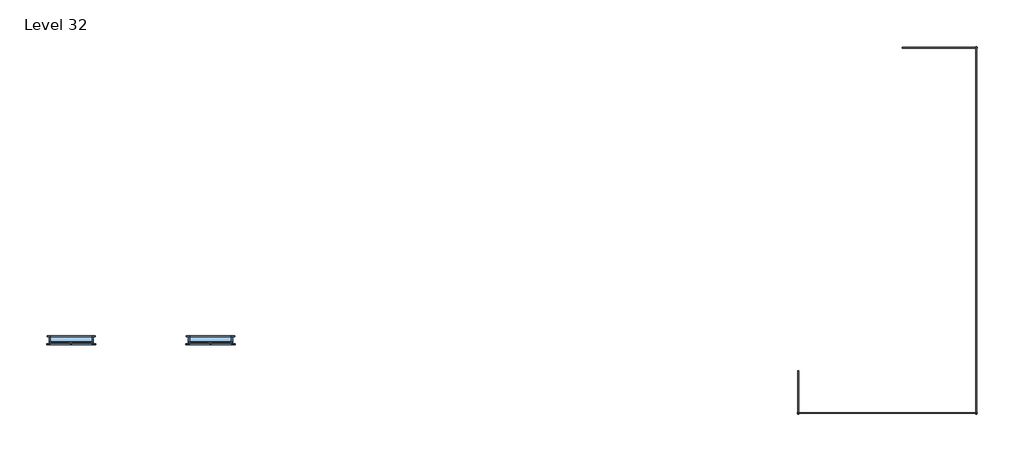
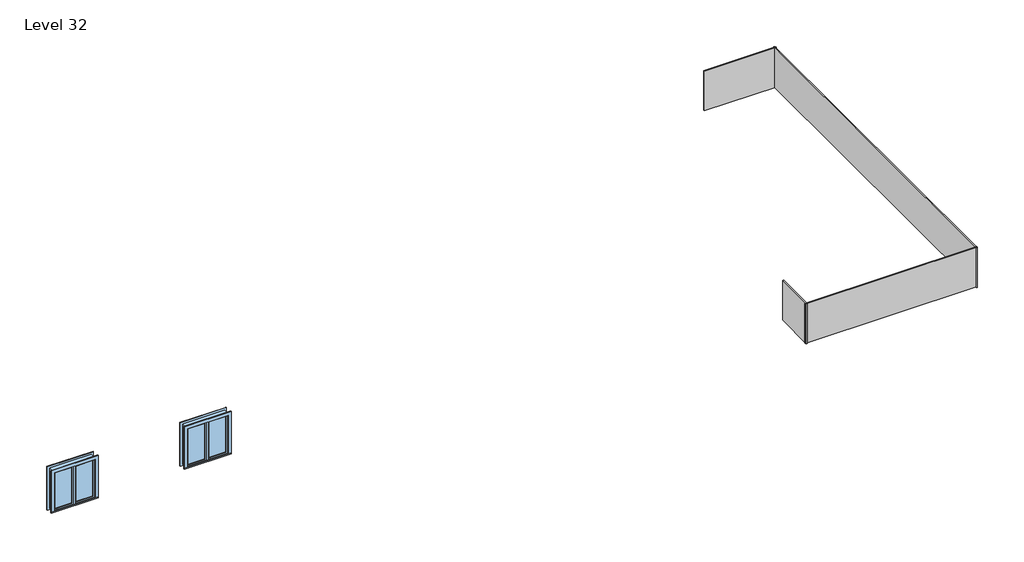
# One storey: 4 plates, 2 windows.
"""IFC4 building model written with IfcOpenShell, lengths in millimetres."""

from ifc_helpers import new_model, si_unit, origin, place, context, project, spatial, transform, mapped, element, save
from components import system_panel_glazed_4fcd3a06, system_panel_glazed_f6fb2dd6, system_panel_glazed_decb64e8, system_panel_glazed_542b97c0, window_0862ab64

model = new_model("IFC4")

# Units and contexts
model_context = context("Model", 3, world=origin())
ifc_project = project(units=[si_unit("LENGTHUNIT", "METRE", prefix="MILLI")], contexts=[model_context])

# Site, building, storey
site = spatial("IfcSite", under=ifc_project)
building = spatial("IfcBuilding", under=site)
storey = spatial("IfcBuildingStorey", under=building, Name="Level 32", Elevation=52197.0)

# Plates
placement = place(None, origin())
system_panel_glazed_shape = system_panel_glazed_4fcd3a06(model_context)
element("IfcPlate", 1, ObjectType="System Panel : Glazed", at=placement, inside=storey, context=model_context, shape_type="MappedRepresentation", body=[
    mapped(system_panel_glazed_shape, transform((9025.4464352, -5860.2278294, 52197.0), x_axis=(-1.0, 0.0, 0.0), y_axis=(0.0, -1.0, 0.0), z_axis=(0.0, 0.0, 1.0))),
])
system_panel_glazed_2_shape = system_panel_glazed_f6fb2dd6(model_context)
element("IfcPlate", 2, ObjectType="System Panel : Glazed", at=placement, inside=storey, context=model_context, shape_type="MappedRepresentation", body=[
    mapped(system_panel_glazed_2_shape, transform((5082.0964352, -15423.3278294, 52197.0), x_axis=(0.0, -1.0, 0.0), y_axis=(1.0, 0.0, 0.0), z_axis=(0.0, 0.0, 1.0))),
])
system_panel_glazed_3_shape = system_panel_glazed_decb64e8(model_context)
element("IfcPlate", 3, ObjectType="System Panel : Glazed", at=placement, inside=storey, context=model_context, shape_type="MappedRepresentation", body=[
    mapped(system_panel_glazed_3_shape, transform((10066.8464352, -10940.2278294, 52197.0), x_axis=(0.0, 1.0, 0.0), y_axis=(-1.0, 0.0, 0.0), z_axis=(0.0, 0.0, 1.0))),
])
system_panel_glazed_4_shape = system_panel_glazed_542b97c0(model_context)
element("IfcPlate", 4, ObjectType="System Panel : Glazed", at=placement, inside=storey, context=model_context, shape_type="MappedRepresentation", body=[
    mapped(system_panel_glazed_4_shape, transform((7574.4714352, -16020.2278294, 52197.0), x_axis=(1.0, 0.0, 0.0), y_axis=(0.0, 1.0, 0.0), z_axis=(0.0, 0.0, 1.0))),
])

# Windows
window_shape = window_0862ab64(model_context)
element("IfcWindow", 5, ObjectType="Casement Dbl with Trim : 48\" x 48\"", at=placement, inside=storey, context=model_context, shape_type="MappedRepresentation", body=[
    mapped(window_shape, transform((-14982.3505427, -13957.4308221, 52197.0), x_axis=(-1.0, 0.0, 0.0), y_axis=(0.0, -1.0, 0.0), z_axis=(0.0, 0.0, 1.0))),
])
element("IfcWindow", 6, ObjectType="Casement Dbl with Trim : 48\" x 48\"", at=placement, inside=storey, context=model_context, shape_type="MappedRepresentation", body=[
    mapped(window_shape, transform((-11129.6382271, -13957.4308221, 52197.0), x_axis=(-1.0, 0.0, 0.0), y_axis=(0.0, -1.0, 0.0), z_axis=(0.0, 0.0, 1.0))),
])

save(model, "model.ifc")

# Revit data of these elements
# Type "System Panel : Glazed"
#   Construction Type Id = "GSP4R"
#   Analytic Construction = "1/8 in Pilkington single glazing"
#   Visual Light Transmittance = 0.9
#   Solar Heat Gain Coefficient = 0.86
#   Heat Transfer Coefficient (U) = 1.18115 BTU/(h·ft²·°F)
# Type "Casement Dbl with Trim : 48\" x 48\""
#   Type Mark = "10"
#   Construction Type Id = "GSP4R"
#   Assembly Code = "B2020100"
#   Analytic Construction = "1/8 in Pilkington single glazing"
#   Visual Light Transmittance = 0.9
#   Solar Heat Gain Coefficient = 0.78
#   Heat Transfer Coefficient (U) = 0.6496 BTU/(h·ft²·°F)
#   Height = 4' - 0"
#   Default Sill Height = 3' - 0"
#   Trim Projection - Ext. = 0' - 0 1/2"
#   Trim Projection - Int. = 0' - 0 3/4"
#   Trim Width - Exterior = 0' - 3 1/2"
#   Trim Width - Interior = 0' - 3 1/2"
#   Width = 4' - 0"
#   Window Inset = 0' - 0 3/4"
#   Define Thermal Properties by = 1
#   Glass Pane Material = Glass
#   Sash Material = Sash
#   Trim Exterior Material = Trim
#   Trim Interior Material = Trim
#   Wall Closure = (empty or 0)
# Elements 1, 2, 3, 4 (IfcPlate, "System Panel : Glazed")
#   Phase Created = New Construction
#   Materials on its faces: "Glass"
# Element 5 (IfcWindow, "Casement Dbl with Trim : 48\" x 48\"")
#   Mark = "15"
#   Phase Created = New Construction
#   Materials on its faces: "Sash", "Trim", "Glass"
# Element 6 (IfcWindow, "Casement Dbl with Trim : 48\" x 48\"")
#   Mark = "16"
#   Phase Created = New Construction
#   Materials on its faces: "Sash", "Trim", "Glass"
# Materials
#   "Glass": class "Glass", colour RGB 0 128 192, transparency 0.75, Description = "Soda Lime Glass", Cost = 0
#   "Sash": class "Wood", colour RGB 224 178 126, transparency 0
#   "Trim": class "Wood", colour RGB 224 178 126, transparency 0
